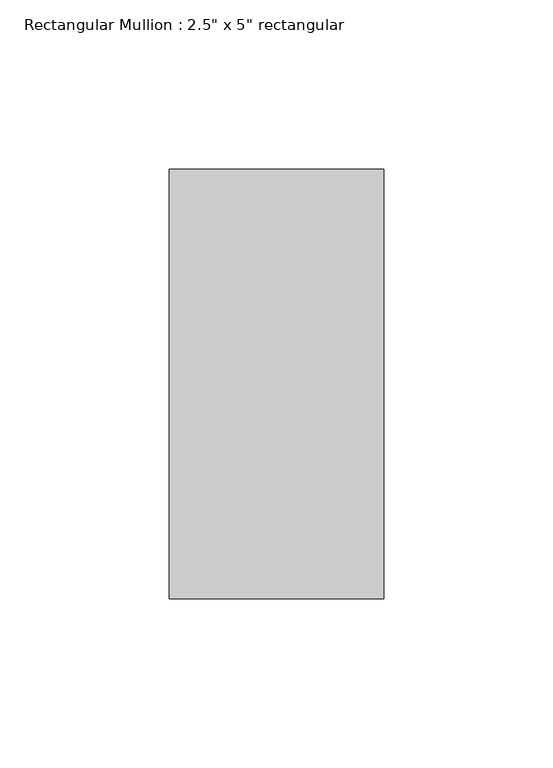
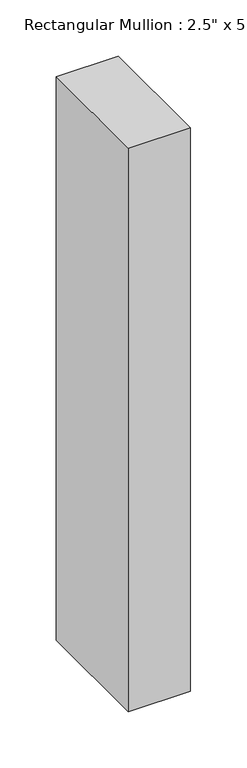
"""IFC4 building model written with IfcOpenShell, lengths in millimetres: member geometry."""

from ifc_helpers import new_model, si_unit, frame, origin, place, context, project, spatial, polyline, outline, extrude, source, transform, mapped, element, save


def member_47bfaf8a(model_context):
    return source(origin(), model_context, "Body", "SweptSolid", [
        extrude(outline(polyline([(0.0, 63.5), (0.0, -63.5), (-63.5, -63.5), (-63.5, 63.5), (0.0, 63.5)])), frame((0.0, 0.0, -609.6), z_axis=(0.0, 0.0, 1.0), x_axis=(1.0, 0.0, 0.0)), (0.0, 0.0, 1.0), 609.6),
    ])


if __name__ == "__main__":
    model = new_model("IFC4")
    model_context = context("Model", 3, world=origin())
    ifc_project = project(units=[si_unit("LENGTHUNIT", "METRE", prefix="MILLI")], contexts=[model_context])
    site = spatial("IfcSite", under=ifc_project)
    building = spatial("IfcBuilding", under=site)
    placement = place(None, origin())
    member_shape = member_47bfaf8a(model_context)
    element("IfcMember", 1, ObjectType="Rectangular Mullion : 2.5\" x 5\" rectangular", at=placement, inside=building, context=model_context, shape_type="MappedRepresentation", body=[
        mapped(member_shape, transform((0.0, 0.0, 0.0), x_axis=(1.0, 0.0, 0.0), y_axis=(0.0, 1.0, 0.0), z_axis=(0.0, 0.0, 1.0))),
    ])
    save(model, "model.ifc")

# Revit data of these elements
# Type "Rectangular Mullion : 2.5\" x 5\" rectangular"
#   built-in parameter 1007304 = 0.416667 (stored number, unit not read)
#   built-in parameter 1007301 = 0.104167 (stored number, unit not read)
#   built-in parameter 1007300 = 0.104167 (stored number, unit not read)
# Element 1 (IfcMember, "Rectangular Mullion : 2.5\" x 5\" rectangular")
#   Materials on its faces: "door colour"
# Materials
#   "door colour": class "Generic", colour RGB 120 120 120, transparency 0, Cost = 0
